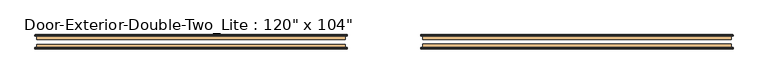
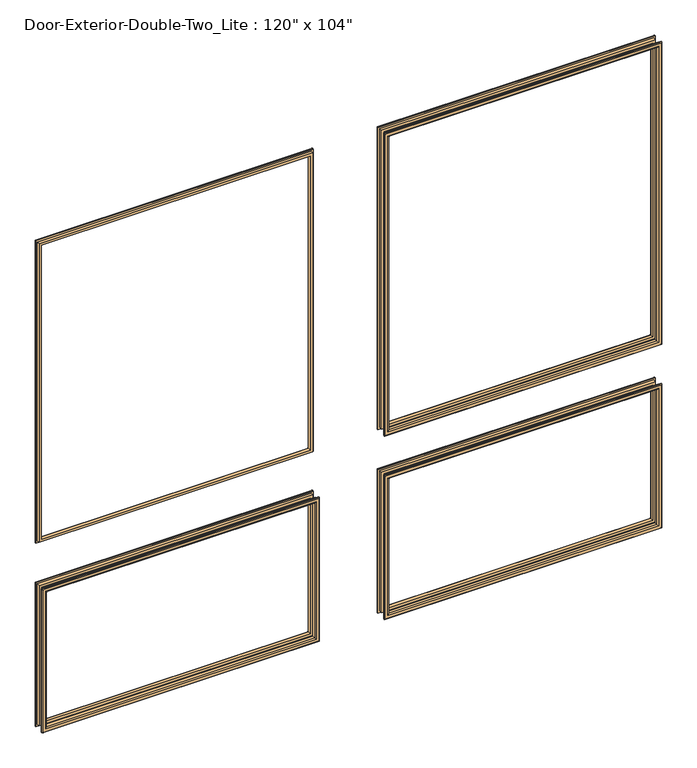
"""IFC4 building model written with IfcOpenShell, lengths in millimetres: door geometry."""

from ifc_helpers import new_model, si_unit, frame, origin, place, context, project, spatial, ellipse_curve, source, transform, mapped, element, save
from ifc_brep_helpers import plane_surface, cylinder_surface, advanced_brep


def door_e43601eb(model_context):
    return source(origin(), model_context, "Body", "AdvancedBrep", [
        advanced_brep(
        [(-1371.6, 69.85, 914.4), (-1371.6, 82.55, 914.4), (-1371.6, 82.55, 254.0), (-1371.6, 69.85, 254.0), (-1359.6, 83.55, 902.4), (-1359.6, 69.85, 902.4), (-1359.6, 69.85, 266.0), (-1359.6, 83.55, 266.0), (-1364.6, 88.55, 907.4), (-1364.6, 88.55, 261.0), (-1379.6, 86.55, 922.4), (-1377.6, 88.55, 920.4), (-1377.6, 88.55, 248.0), (-1379.6, 86.55, 246.0), (-1379.6, 82.55, 922.4), (-1379.6, 82.55, 246.0), (-152.4, 82.55, 254.0), (-152.4, 69.85, 254.0), (-164.4, 69.85, 266.0), (-164.4, 83.55, 266.0), (-159.4, 88.55, 261.0), (-146.4, 88.55, 248.0), (-144.4, 86.55, 246.0), (-144.4, 82.55, 246.0), (-152.4, 82.55, 914.4), (-152.4, 69.85, 914.4), (-164.4, 69.85, 902.4), (-164.4, 83.55, 902.4), (-159.4, 88.55, 907.4), (-146.4, 88.55, 920.4), (-144.4, 86.55, 922.4), (-144.4, 82.55, 922.4)],
        [
            (0, 1),
            (1, 2),
            (2, 3),
            (3, 0),
            (4, 5),
            (5, 6),
            (6, 7),
            (7, 4),
            (8, 4, ellipse_curve(frame((-1364.6, 83.55, 907.4), z_axis=(-0.7071067811865475, 0.0, -0.7071067811865475), x_axis=(-0.7071067811865474, 0.0, 0.7071067811865476)), 7.0710678, 5.0)),
            (7, 9, ellipse_curve(frame((-1364.6, 83.55, 261.0), z_axis=(-0.7071067811865475, 0.0, 0.7071067811865475), x_axis=(0.7071067811865474, 0.0, 0.7071067811865476)), 7.0710678, 5.0)),
            (9, 8),
            (10, 11, ellipse_curve(frame((-1377.6, 86.55, 920.4), z_axis=(-0.7071067811865475, 0.0, -0.7071067811865475), x_axis=(-0.7071067811865474, 0.0, 0.7071067811865476)), 2.8284271, 2.0)),
            (11, 12),
            (12, 13, ellipse_curve(frame((-1377.6, 86.55, 248.0), z_axis=(-0.7071067811865475, 0.0, 0.7071067811865475), x_axis=(0.7071067811865474, 0.0, 0.7071067811865476)), 2.8284271, 2.0)),
            (13, 10),
            (14, 10),
            (13, 15),
            (15, 14),
            (2, 16),
            (16, 17),
            (17, 3),
            (6, 18),
            (18, 19),
            (19, 7),
            (19, 20, ellipse_curve(frame((-159.4, 83.55, 261.0), z_axis=(-0.7071067811865475, 0.0, -0.7071067811865475), x_axis=(-0.7071067811865476, 0.0, 0.7071067811865474)), 7.0710678, 5.0)),
            (20, 9),
            (12, 21),
            (21, 22, ellipse_curve(frame((-146.4, 86.55, 248.0), z_axis=(-0.7071067811865475, 0.0, -0.7071067811865475), x_axis=(-0.7071067811865476, 0.0, 0.7071067811865474)), 2.8284271, 2.0)),
            (22, 13),
            (22, 23),
            (23, 15),
            (16, 24),
            (24, 25),
            (25, 17),
            (18, 26),
            (26, 27),
            (27, 19),
            (27, 28, ellipse_curve(frame((-159.4, 83.55, 907.4), z_axis=(0.7071067811865475, 0.0, -0.7071067811865475), x_axis=(-0.7071067811865474, 0.0, -0.7071067811865476)), 7.0710678, 5.0)),
            (28, 20),
            (21, 29),
            (29, 30, ellipse_curve(frame((-146.4, 86.55, 920.4), z_axis=(0.7071067811865475, 0.0, -0.7071067811865475), x_axis=(-0.7071067811865474, 0.0, -0.7071067811865476)), 2.8284271, 2.0)),
            (30, 22),
            (30, 31),
            (31, 23),
            (31, 14),
            (1, 24),
            (0, 25),
            (5, 26),
            (4, 27),
            (8, 28),
            (11, 29),
            (10, 30),
        ],
        [
            plane_surface(frame((-1371.6, 82.55, 914.4), z_axis=(-1.0, 0.0, 0.0), x_axis=(0.0, 0.0, -1.0))),
            plane_surface(frame((-1359.6, 69.85, 902.4), z_axis=(1.0, 0.0, 0.0), x_axis=(0.0, 0.0, -1.0))),
            cylinder_surface(frame((-1364.6, 83.55, 914.4), z_axis=(0.0, 0.0, 1.0), x_axis=(-1.0, 0.0, 0.0)), 5.0),
            cylinder_surface(frame((-1377.6, 86.55, 914.4), z_axis=(0.0, 0.0, 1.0), x_axis=(-1.0, 0.0, 0.0)), 2.0),
            plane_surface(frame((-1379.6, 86.55, 922.4), z_axis=(-1.0, 0.0, 0.0), x_axis=(0.0, 0.0, -1.0))),
            plane_surface(frame((-1371.6, 82.55, 254.0), z_axis=(0.0, 0.0, -1.0), x_axis=(1.0, 0.0, 0.0))),
            plane_surface(frame((-1359.6, 69.85, 266.0), z_axis=(0.0, 0.0, 1.0), x_axis=(1.0, 0.0, 0.0))),
            cylinder_surface(frame((-1371.6, 83.55, 261.0), z_axis=(-1.0, 0.0, 0.0), x_axis=(0.0, 0.0, -1.0)), 5.0),
            cylinder_surface(frame((-1371.6, 86.55, 248.0), z_axis=(-1.0, 0.0, 0.0), x_axis=(0.0, 0.0, -1.0)), 2.0),
            plane_surface(frame((-1379.6, 86.55, 246.0), z_axis=(0.0, 0.0, -1.0), x_axis=(1.0, 0.0, 0.0))),
            plane_surface(frame((-152.4, 82.55, 254.0), z_axis=(1.0, 0.0, 0.0), x_axis=(0.0, 0.0, 1.0))),
            plane_surface(frame((-164.4, 69.85, 266.0), z_axis=(-1.0, 0.0, 0.0), x_axis=(0.0, 0.0, 1.0))),
            cylinder_surface(frame((-159.4, 83.55, 254.0), z_axis=(0.0, 0.0, -1.0), x_axis=(1.0, 0.0, 0.0)), 5.0),
            cylinder_surface(frame((-146.4, 86.55, 254.0), z_axis=(0.0, 0.0, -1.0), x_axis=(1.0, 0.0, 0.0)), 2.0),
            plane_surface(frame((-144.4, 86.55, 246.0), z_axis=(1.0, 0.0, 0.0), x_axis=(0.0, 0.0, 1.0))),
            plane_surface(frame((-144.4, 82.55, 922.4), z_axis=(0.0, -1.0, 0.0), x_axis=(-1.0, 0.0, 0.0))),
            plane_surface(frame((-152.4, 82.55, 914.4), z_axis=(0.0, 0.0, 1.0), x_axis=(-1.0, 0.0, 0.0))),
            plane_surface(frame((-152.4, 69.85, 914.4), z_axis=(0.0, -1.0, 0.0), x_axis=(-1.0, 0.0, 0.0))),
            plane_surface(frame((-164.4, 69.85, 902.4), z_axis=(0.0, 0.0, -1.0), x_axis=(-1.0, 0.0, 0.0))),
            cylinder_surface(frame((-152.4, 83.55, 907.4), z_axis=(1.0, 0.0, 0.0), x_axis=(0.0, 0.0, 1.0)), 5.0),
            plane_surface(frame((-159.4, 88.55, 907.4), z_axis=(0.0, 1.0, 0.0), x_axis=(-1.0, 0.0, 0.0))),
            cylinder_surface(frame((-152.4, 86.55, 920.4), z_axis=(1.0, 0.0, 0.0), x_axis=(0.0, 0.0, 1.0)), 2.0),
            plane_surface(frame((-144.4, 86.55, 922.4), z_axis=(0.0, 0.0, 1.0), x_axis=(-1.0, 0.0, 0.0))),
        ],
        [
            (0, [[1, 2, 3, 4]]),
            (1, [[5, 6, 7, 8]]),
            (2, [[9, -8, 10, 11]]),
            (3, [[12, 13, 14, 15]]),
            (4, [[16, -15, 17, 18]]),
            (5, [[-3, 19, 20, 21]]),
            (6, [[-7, 22, 23, 24]]),
            (7, [[-10, -24, 25, 26]]),
            (8, [[-14, 27, 28, 29]]),
            (9, [[-17, -29, 30, 31]]),
            (10, [[-20, 32, 33, 34]]),
            (11, [[-23, 35, 36, 37]]),
            (12, [[-25, -37, 38, 39]]),
            (13, [[-28, 40, 41, 42]]),
            (14, [[-30, -42, 43, 44]]),
            (15, [[-31, -44, 45, -18], [46, -32, -19, -2]]),
            (16, [[-33, -46, -1, 47]]),
            (17, [[-21, -34, -47, -4], [48, -35, -22, -6]]),
            (18, [[-36, -48, -5, 49]]),
            (19, [[-38, -49, -9, 50]]),
            (20, [[51, -40, -27, -13], [-26, -39, -50, -11]]),
            (21, [[-41, -51, -12, 52]]),
            (22, [[-43, -52, -16, -45]]),
        ],
    ),
        advanced_brep(
        [(152.4, 69.85, 914.4), (152.4, 82.55, 914.4), (152.4, 82.55, 254.0), (152.4, 69.85, 254.0), (164.4, 83.55, 902.4), (164.4, 69.85, 902.4), (164.4, 69.85, 266.0), (164.4, 83.55, 266.0), (159.4, 88.55, 907.4), (159.4, 88.55, 261.0), (144.4, 86.55, 922.4), (146.4, 88.55, 920.4), (146.4, 88.55, 248.0), (144.4, 86.55, 246.0), (144.4, 82.55, 922.4), (144.4, 82.55, 246.0), (1371.6, 82.55, 254.0), (1371.6, 69.85, 254.0), (1359.6, 69.85, 266.0), (1359.6, 83.55, 266.0), (1364.6, 88.55, 261.0), (1377.6, 88.55, 248.0), (1379.6, 86.55, 246.0), (1379.6, 82.55, 246.0), (1371.6, 82.55, 914.4), (1371.6, 69.85, 914.4), (1359.6, 69.85, 902.4), (1359.6, 83.55, 902.4), (1364.6, 88.55, 907.4), (1377.6, 88.55, 920.4), (1379.6, 86.55, 922.4), (1379.6, 82.55, 922.4)],
        [
            (0, 1),
            (1, 2),
            (2, 3),
            (3, 0),
            (4, 5),
            (5, 6),
            (6, 7),
            (7, 4),
            (8, 4, ellipse_curve(frame((159.4, 83.55, 907.4), z_axis=(-0.7071067811865475, 0.0, -0.7071067811865475), x_axis=(-0.7071067811865474, 0.0, 0.7071067811865476)), 7.0710678, 5.0)),
            (7, 9, ellipse_curve(frame((159.4, 83.55, 261.0), z_axis=(-0.7071067811865475, 0.0, 0.7071067811865475), x_axis=(0.7071067811865474, 0.0, 0.7071067811865476)), 7.0710678, 5.0)),
            (9, 8),
            (10, 11, ellipse_curve(frame((146.4, 86.55, 920.4), z_axis=(-0.7071067811865475, 0.0, -0.7071067811865475), x_axis=(-0.7071067811865474, 0.0, 0.7071067811865476)), 2.8284271, 2.0)),
            (11, 12),
            (12, 13, ellipse_curve(frame((146.4, 86.55, 248.0), z_axis=(-0.7071067811865475, 0.0, 0.7071067811865475), x_axis=(0.7071067811865474, 0.0, 0.7071067811865476)), 2.8284271, 2.0)),
            (13, 10),
            (14, 10),
            (13, 15),
            (15, 14),
            (2, 16),
            (16, 17),
            (17, 3),
            (6, 18),
            (18, 19),
            (19, 7),
            (19, 20, ellipse_curve(frame((1364.6, 83.55, 261.0), z_axis=(-0.7071067811865475, 0.0, -0.7071067811865475), x_axis=(-0.7071067811865476, 0.0, 0.7071067811865474)), 7.0710678, 5.0)),
            (20, 9),
            (12, 21),
            (21, 22, ellipse_curve(frame((1377.6, 86.55, 248.0), z_axis=(-0.7071067811865475, 0.0, -0.7071067811865475), x_axis=(-0.7071067811865476, 0.0, 0.7071067811865474)), 2.8284271, 2.0)),
            (22, 13),
            (22, 23),
            (23, 15),
            (16, 24),
            (24, 25),
            (25, 17),
            (18, 26),
            (26, 27),
            (27, 19),
            (27, 28, ellipse_curve(frame((1364.6, 83.55, 907.4), z_axis=(0.7071067811865475, 0.0, -0.7071067811865475), x_axis=(-0.7071067811865474, 0.0, -0.7071067811865476)), 7.0710678, 5.0)),
            (28, 20),
            (21, 29),
            (29, 30, ellipse_curve(frame((1377.6, 86.55, 920.4), z_axis=(0.7071067811865475, 0.0, -0.7071067811865475), x_axis=(-0.7071067811865474, 0.0, -0.7071067811865476)), 2.8284271, 2.0)),
            (30, 22),
            (30, 31),
            (31, 23),
            (31, 14),
            (1, 24),
            (0, 25),
            (5, 26),
            (4, 27),
            (8, 28),
            (11, 29),
            (10, 30),
        ],
        [
            plane_surface(frame((152.4, 82.55, 914.4), z_axis=(-1.0, 0.0, 0.0), x_axis=(0.0, 0.0, -1.0))),
            plane_surface(frame((164.4, 69.85, 902.4), z_axis=(1.0, 0.0, 0.0), x_axis=(0.0, 0.0, -1.0))),
            cylinder_surface(frame((159.4, 83.55, 914.4), z_axis=(0.0, 0.0, 1.0), x_axis=(-1.0, 0.0, 0.0)), 5.0),
            cylinder_surface(frame((146.4, 86.55, 914.4), z_axis=(0.0, 0.0, 1.0), x_axis=(-1.0, 0.0, 0.0)), 2.0),
            plane_surface(frame((144.4, 86.55, 922.4), z_axis=(-1.0, 0.0, 0.0), x_axis=(0.0, 0.0, -1.0))),
            plane_surface(frame((152.4, 82.55, 254.0), z_axis=(0.0, 0.0, -1.0), x_axis=(1.0, 0.0, 0.0))),
            plane_surface(frame((164.4, 69.85, 266.0), z_axis=(0.0, 0.0, 1.0), x_axis=(1.0, 0.0, 0.0))),
            cylinder_surface(frame((152.4, 83.55, 261.0), z_axis=(-1.0, 0.0, 0.0), x_axis=(0.0, 0.0, -1.0)), 5.0),
            cylinder_surface(frame((152.4, 86.55, 248.0), z_axis=(-1.0, 0.0, 0.0), x_axis=(0.0, 0.0, -1.0)), 2.0),
            plane_surface(frame((144.4, 86.55, 246.0), z_axis=(0.0, 0.0, -1.0), x_axis=(1.0, 0.0, 0.0))),
            plane_surface(frame((1371.6, 82.55, 254.0), z_axis=(1.0, 0.0, 0.0), x_axis=(0.0, 0.0, 1.0))),
            plane_surface(frame((1359.6, 69.85, 266.0), z_axis=(-1.0, 0.0, 0.0), x_axis=(0.0, 0.0, 1.0))),
            cylinder_surface(frame((1364.6, 83.55, 254.0), z_axis=(0.0, 0.0, -1.0), x_axis=(1.0, 0.0, 0.0)), 5.0),
            cylinder_surface(frame((1377.6, 86.55, 254.0), z_axis=(0.0, 0.0, -1.0), x_axis=(1.0, 0.0, 0.0)), 2.0),
            plane_surface(frame((1379.6, 86.55, 246.0), z_axis=(1.0, 0.0, 0.0), x_axis=(0.0, 0.0, 1.0))),
            plane_surface(frame((1379.6, 82.55, 922.4), z_axis=(0.0, -1.0, 0.0), x_axis=(-1.0, 0.0, 0.0))),
            plane_surface(frame((1371.6, 82.55, 914.4), z_axis=(0.0, 0.0, 1.0), x_axis=(-1.0, 0.0, 0.0))),
            plane_surface(frame((1371.6, 69.85, 914.4), z_axis=(0.0, -1.0, 0.0), x_axis=(-1.0, 0.0, 0.0))),
            plane_surface(frame((1359.6, 69.85, 902.4), z_axis=(0.0, 0.0, -1.0), x_axis=(-1.0, 0.0, 0.0))),
            cylinder_surface(frame((1371.6, 83.55, 907.4), z_axis=(1.0, 0.0, 0.0), x_axis=(0.0, 0.0, 1.0)), 5.0),
            plane_surface(frame((1364.6, 88.55, 907.4), z_axis=(0.0, 1.0, 0.0), x_axis=(-1.0, 0.0, 0.0))),
            cylinder_surface(frame((1371.6, 86.55, 920.4), z_axis=(1.0, 0.0, 0.0), x_axis=(0.0, 0.0, 1.0)), 2.0),
            plane_surface(frame((1379.6, 86.55, 922.4), z_axis=(0.0, 0.0, 1.0), x_axis=(-1.0, 0.0, 0.0))),
        ],
        [
            (0, [[1, 2, 3, 4]]),
            (1, [[5, 6, 7, 8]]),
            (2, [[9, -8, 10, 11]]),
            (3, [[12, 13, 14, 15]]),
            (4, [[16, -15, 17, 18]]),
            (5, [[-3, 19, 20, 21]]),
            (6, [[-7, 22, 23, 24]]),
            (7, [[-10, -24, 25, 26]]),
            (8, [[-14, 27, 28, 29]]),
            (9, [[-17, -29, 30, 31]]),
            (10, [[-20, 32, 33, 34]]),
            (11, [[-23, 35, 36, 37]]),
            (12, [[-25, -37, 38, 39]]),
            (13, [[-28, 40, 41, 42]]),
            (14, [[-30, -42, 43, 44]]),
            (15, [[-31, -44, 45, -18], [46, -32, -19, -2]]),
            (16, [[-33, -46, -1, 47]]),
            (17, [[-21, -34, -47, -4], [48, -35, -22, -6]]),
            (18, [[-36, -48, -5, 49]]),
            (19, [[-38, -49, -9, 50]]),
            (20, [[51, -40, -27, -13], [-26, -39, -50, -11]]),
            (21, [[-41, -51, -12, 52]]),
            (22, [[-43, -52, -16, -45]]),
        ],
    ),
        advanced_brep(
        [(152.4, 69.85, 2524.125), (152.4, 82.55, 2524.125), (152.4, 82.55, 1117.6), (152.4, 69.85, 1117.6), (164.4, 83.55, 2512.125), (164.4, 69.85, 2512.125), (164.4, 69.85, 1129.6), (164.4, 83.55, 1129.6), (159.4, 88.55, 2517.125), (159.4, 88.55, 1124.6), (144.4, 86.55, 2532.125), (146.4, 88.55, 2530.125), (146.4, 88.55, 1111.6), (144.4, 86.55, 1109.6), (144.4, 82.55, 2532.125), (144.4, 82.55, 1109.6), (1371.6, 82.55, 1117.6), (1371.6, 69.85, 1117.6), (1359.6, 69.85, 1129.6), (1359.6, 83.55, 1129.6), (1364.6, 88.55, 1124.6), (1377.6, 88.55, 1111.6), (1379.6, 86.55, 1109.6), (1379.6, 82.55, 1109.6), (1371.6, 82.55, 2524.125), (1371.6, 69.85, 2524.125), (1359.6, 69.85, 2512.125), (1359.6, 83.55, 2512.125), (1364.6, 88.55, 2517.125), (1377.6, 88.55, 2530.125), (1379.6, 86.55, 2532.125), (1379.6, 82.55, 2532.125)],
        [
            (0, 1),
            (1, 2),
            (2, 3),
            (3, 0),
            (4, 5),
            (5, 6),
            (6, 7),
            (7, 4),
            (8, 4, ellipse_curve(frame((159.4, 83.55, 2517.125), z_axis=(-0.7071067811865475, 0.0, -0.7071067811865475), x_axis=(-0.7071067811865474, 0.0, 0.7071067811865476)), 7.0710678, 5.0)),
            (7, 9, ellipse_curve(frame((159.4, 83.55, 1124.6), z_axis=(-0.7071067811865475, 0.0, 0.7071067811865475), x_axis=(0.7071067811865474, 0.0, 0.7071067811865476)), 7.0710678, 5.0)),
            (9, 8),
            (10, 11, ellipse_curve(frame((146.4, 86.55, 2530.125), z_axis=(-0.7071067811865475, 0.0, -0.7071067811865475), x_axis=(-0.7071067811865474, 0.0, 0.7071067811865476)), 2.8284271, 2.0)),
            (11, 12),
            (12, 13, ellipse_curve(frame((146.4, 86.55, 1111.6), z_axis=(-0.7071067811865475, 0.0, 0.7071067811865475), x_axis=(0.7071067811865474, 0.0, 0.7071067811865476)), 2.8284271, 2.0)),
            (13, 10),
            (14, 10),
            (13, 15),
            (15, 14),
            (2, 16),
            (16, 17),
            (17, 3),
            (6, 18),
            (18, 19),
            (19, 7),
            (19, 20, ellipse_curve(frame((1364.6, 83.55, 1124.6), z_axis=(-0.7071067811865475, 0.0, -0.7071067811865475), x_axis=(-0.7071067811865476, 0.0, 0.7071067811865474)), 7.0710678, 5.0)),
            (20, 9),
            (12, 21),
            (21, 22, ellipse_curve(frame((1377.6, 86.55, 1111.6), z_axis=(-0.7071067811865475, 0.0, -0.7071067811865475), x_axis=(-0.7071067811865476, 0.0, 0.7071067811865474)), 2.8284271, 2.0)),
            (22, 13),
            (22, 23),
            (23, 15),
            (16, 24),
            (24, 25),
            (25, 17),
            (18, 26),
            (26, 27),
            (27, 19),
            (27, 28, ellipse_curve(frame((1364.6, 83.55, 2517.125), z_axis=(0.7071067811865475, 0.0, -0.7071067811865475), x_axis=(-0.7071067811865474, 0.0, -0.7071067811865476)), 7.0710678, 5.0)),
            (28, 20),
            (21, 29),
            (29, 30, ellipse_curve(frame((1377.6, 86.55, 2530.125), z_axis=(0.7071067811865475, 0.0, -0.7071067811865475), x_axis=(-0.7071067811865474, 0.0, -0.7071067811865476)), 2.8284271, 2.0)),
            (30, 22),
            (30, 31),
            (31, 23),
            (31, 14),
            (1, 24),
            (0, 25),
            (5, 26),
            (4, 27),
            (8, 28),
            (11, 29),
            (10, 30),
        ],
        [
            plane_surface(frame((152.4, 82.55, 2524.125), z_axis=(-1.0, 0.0, 0.0), x_axis=(0.0, 0.0, -1.0))),
            plane_surface(frame((164.4, 69.85, 2512.125), z_axis=(1.0, 0.0, 0.0), x_axis=(0.0, 0.0, -1.0))),
            cylinder_surface(frame((159.4, 83.55, 2524.125), z_axis=(0.0, 0.0, 1.0), x_axis=(-1.0, 0.0, 0.0)), 5.0),
            cylinder_surface(frame((146.4, 86.55, 2524.125), z_axis=(0.0, 0.0, 1.0), x_axis=(-1.0, 0.0, 0.0)), 2.0),
            plane_surface(frame((144.4, 86.55, 2532.125), z_axis=(-1.0, 0.0, 0.0), x_axis=(0.0, 0.0, -1.0))),
            plane_surface(frame((152.4, 82.55, 1117.6), z_axis=(0.0, 0.0, -1.0), x_axis=(1.0, 0.0, 0.0))),
            plane_surface(frame((164.4, 69.85, 1129.6), z_axis=(0.0, 0.0, 1.0), x_axis=(1.0, 0.0, 0.0))),
            cylinder_surface(frame((152.4, 83.55, 1124.6), z_axis=(-1.0, 0.0, 0.0), x_axis=(0.0, 0.0, -1.0)), 5.0),
            cylinder_surface(frame((152.4, 86.55, 1111.6), z_axis=(-1.0, 0.0, 0.0), x_axis=(0.0, 0.0, -1.0)), 2.0),
            plane_surface(frame((144.4, 86.55, 1109.6), z_axis=(0.0, 0.0, -1.0), x_axis=(1.0, 0.0, 0.0))),
            plane_surface(frame((1371.6, 82.55, 1117.6), z_axis=(1.0, 0.0, 0.0), x_axis=(0.0, 0.0, 1.0))),
            plane_surface(frame((1359.6, 69.85, 1129.6), z_axis=(-1.0, 0.0, 0.0), x_axis=(0.0, 0.0, 1.0))),
            cylinder_surface(frame((1364.6, 83.55, 1117.6), z_axis=(0.0, 0.0, -1.0), x_axis=(1.0, 0.0, 0.0)), 5.0),
            cylinder_surface(frame((1377.6, 86.55, 1117.6), z_axis=(0.0, 0.0, -1.0), x_axis=(1.0, 0.0, 0.0)), 2.0),
            plane_surface(frame((1379.6, 86.55, 1109.6), z_axis=(1.0, 0.0, 0.0), x_axis=(0.0, 0.0, 1.0))),
            plane_surface(frame((1379.6, 82.55, 2532.125), z_axis=(0.0, -1.0, 0.0), x_axis=(-1.0, 0.0, 0.0))),
            plane_surface(frame((1371.6, 82.55, 2524.125), z_axis=(0.0, 0.0, 1.0), x_axis=(-1.0, 0.0, 0.0))),
            plane_surface(frame((1371.6, 69.85, 2524.125), z_axis=(0.0, -1.0, 0.0), x_axis=(-1.0, 0.0, 0.0))),
            plane_surface(frame((1359.6, 69.85, 2512.125), z_axis=(0.0, 0.0, -1.0), x_axis=(-1.0, 0.0, 0.0))),
            cylinder_surface(frame((1371.6, 83.55, 2517.125), z_axis=(1.0, 0.0, 0.0), x_axis=(0.0, 0.0, 1.0)), 5.0),
            plane_surface(frame((1364.6, 88.55, 2517.125), z_axis=(0.0, 1.0, 0.0), x_axis=(-1.0, 0.0, 0.0))),
            cylinder_surface(frame((1371.6, 86.55, 2530.125), z_axis=(1.0, 0.0, 0.0), x_axis=(0.0, 0.0, 1.0)), 2.0),
            plane_surface(frame((1379.6, 86.55, 2532.125), z_axis=(0.0, 0.0, 1.0), x_axis=(-1.0, 0.0, 0.0))),
        ],
        [
            (0, [[1, 2, 3, 4]]),
            (1, [[5, 6, 7, 8]]),
            (2, [[9, -8, 10, 11]]),
            (3, [[12, 13, 14, 15]]),
            (4, [[16, -15, 17, 18]]),
            (5, [[-3, 19, 20, 21]]),
            (6, [[-7, 22, 23, 24]]),
            (7, [[-10, -24, 25, 26]]),
            (8, [[-14, 27, 28, 29]]),
            (9, [[-17, -29, 30, 31]]),
            (10, [[-20, 32, 33, 34]]),
            (11, [[-23, 35, 36, 37]]),
            (12, [[-25, -37, 38, 39]]),
            (13, [[-28, 40, 41, 42]]),
            (14, [[-30, -42, 43, 44]]),
            (15, [[-31, -44, 45, -18], [46, -32, -19, -2]]),
            (16, [[-33, -46, -1, 47]]),
            (17, [[-21, -34, -47, -4], [48, -35, -22, -6]]),
            (18, [[-36, -48, -5, 49]]),
            (19, [[-38, -49, -9, 50]]),
            (20, [[51, -40, -27, -13], [-26, -39, -50, -11]]),
            (21, [[-41, -51, -12, 52]]),
            (22, [[-43, -52, -16, -45]]),
        ],
    ),
        advanced_brep(
        [(-1371.6, 69.85, 2524.125), (-1371.6, 82.55, 2524.125), (-1371.6, 82.55, 1117.6), (-1371.6, 69.85, 1117.6), (-1359.6, 83.55, 2512.125), (-1359.6, 69.85, 2512.125), (-1359.6, 69.85, 1129.6), (-1359.6, 83.55, 1129.6), (-1364.6, 88.55, 2517.125), (-1364.6, 88.55, 1124.6), (-1379.6, 86.55, 2532.125), (-1377.6, 88.55, 2530.125), (-1377.6, 88.55, 1111.6), (-1379.6, 86.55, 1109.6), (-1379.6, 82.55, 2532.125), (-1379.6, 82.55, 1109.6), (-152.4, 82.55, 1117.6), (-152.4, 69.85, 1117.6), (-164.4, 69.85, 1129.6), (-164.4, 83.55, 1129.6), (-159.4, 88.55, 1124.6), (-146.4, 88.55, 1111.6), (-144.4, 86.55, 1109.6), (-144.4, 82.55, 1109.6), (-152.4, 82.55, 2524.125), (-152.4, 69.85, 2524.125), (-164.4, 69.85, 2512.125), (-164.4, 83.55, 2512.125), (-159.4, 88.55, 2517.125), (-146.4, 88.55, 2530.125), (-144.4, 86.55, 2532.125), (-144.4, 82.55, 2532.125)],
        [
            (0, 1),
            (1, 2),
            (2, 3),
            (3, 0),
            (4, 5),
            (5, 6),
            (6, 7),
            (7, 4),
            (8, 4, ellipse_curve(frame((-1364.6, 83.55, 2517.125), z_axis=(-0.7071067811865475, 0.0, -0.7071067811865475), x_axis=(-0.7071067811865474, 0.0, 0.7071067811865476)), 7.0710678, 5.0)),
            (7, 9, ellipse_curve(frame((-1364.6, 83.55, 1124.6), z_axis=(-0.7071067811865475, 0.0, 0.7071067811865475), x_axis=(0.7071067811865474, 0.0, 0.7071067811865476)), 7.0710678, 5.0)),
            (9, 8),
            (10, 11, ellipse_curve(frame((-1377.6, 86.55, 2530.125), z_axis=(-0.7071067811865475, 0.0, -0.7071067811865475), x_axis=(-0.7071067811865474, 0.0, 0.7071067811865476)), 2.8284271, 2.0)),
            (11, 12),
            (12, 13, ellipse_curve(frame((-1377.6, 86.55, 1111.6), z_axis=(-0.7071067811865475, 0.0, 0.7071067811865475), x_axis=(0.7071067811865474, 0.0, 0.7071067811865476)), 2.8284271, 2.0)),
            (13, 10),
            (14, 10),
            (13, 15),
            (15, 14),
            (2, 16),
            (16, 17),
            (17, 3),
            (6, 18),
            (18, 19),
            (19, 7),
            (19, 20, ellipse_curve(frame((-159.4, 83.55, 1124.6), z_axis=(-0.7071067811865475, 0.0, -0.7071067811865475), x_axis=(-0.7071067811865476, 0.0, 0.7071067811865474)), 7.0710678, 5.0)),
            (20, 9),
            (12, 21),
            (21, 22, ellipse_curve(frame((-146.4, 86.55, 1111.6), z_axis=(-0.7071067811865475, 0.0, -0.7071067811865475), x_axis=(-0.7071067811865476, 0.0, 0.7071067811865474)), 2.8284271, 2.0)),
            (22, 13),
            (22, 23),
            (23, 15),
            (16, 24),
            (24, 25),
            (25, 17),
            (18, 26),
            (26, 27),
            (27, 19),
            (27, 28, ellipse_curve(frame((-159.4, 83.55, 2517.125), z_axis=(0.7071067811865475, 0.0, -0.7071067811865475), x_axis=(-0.7071067811865474, 0.0, -0.7071067811865476)), 7.0710678, 5.0)),
            (28, 20),
            (21, 29),
            (29, 30, ellipse_curve(frame((-146.4, 86.55, 2530.125), z_axis=(0.7071067811865475, 0.0, -0.7071067811865475), x_axis=(-0.7071067811865474, 0.0, -0.7071067811865476)), 2.8284271, 2.0)),
            (30, 22),
            (30, 31),
            (31, 23),
            (31, 14),
            (1, 24),
            (0, 25),
            (5, 26),
            (4, 27),
            (8, 28),
            (11, 29),
            (10, 30),
        ],
        [
            plane_surface(frame((-1371.6, 82.55, 2524.125), z_axis=(-1.0, 0.0, 0.0), x_axis=(0.0, 0.0, -1.0))),
            plane_surface(frame((-1359.6, 69.85, 2512.125), z_axis=(1.0, 0.0, 0.0), x_axis=(0.0, 0.0, -1.0))),
            cylinder_surface(frame((-1364.6, 83.55, 2524.125), z_axis=(0.0, 0.0, 1.0), x_axis=(-1.0, 0.0, 0.0)), 5.0),
            cylinder_surface(frame((-1377.6, 86.55, 2524.125), z_axis=(0.0, 0.0, 1.0), x_axis=(-1.0, 0.0, 0.0)), 2.0),
            plane_surface(frame((-1379.6, 86.55, 2532.125), z_axis=(-1.0, 0.0, 0.0), x_axis=(0.0, 0.0, -1.0))),
            plane_surface(frame((-1371.6, 82.55, 1117.6), z_axis=(0.0, 0.0, -1.0), x_axis=(1.0, 0.0, 0.0))),
            plane_surface(frame((-1359.6, 69.85, 1129.6), z_axis=(0.0, 0.0, 1.0), x_axis=(1.0, 0.0, 0.0))),
            cylinder_surface(frame((-1371.6, 83.55, 1124.6), z_axis=(-1.0, 0.0, 0.0), x_axis=(0.0, 0.0, -1.0)), 5.0),
            cylinder_surface(frame((-1371.6, 86.55, 1111.6), z_axis=(-1.0, 0.0, 0.0), x_axis=(0.0, 0.0, -1.0)), 2.0),
            plane_surface(frame((-1379.6, 86.55, 1109.6), z_axis=(0.0, 0.0, -1.0), x_axis=(1.0, 0.0, 0.0))),
            plane_surface(frame((-152.4, 82.55, 1117.6), z_axis=(1.0, 0.0, 0.0), x_axis=(0.0, 0.0, 1.0))),
            plane_surface(frame((-164.4, 69.85, 1129.6), z_axis=(-1.0, 0.0, 0.0), x_axis=(0.0, 0.0, 1.0))),
            cylinder_surface(frame((-159.4, 83.55, 1117.6), z_axis=(0.0, 0.0, -1.0), x_axis=(1.0, 0.0, 0.0)), 5.0),
            cylinder_surface(frame((-146.4, 86.55, 1117.6), z_axis=(0.0, 0.0, -1.0), x_axis=(1.0, 0.0, 0.0)), 2.0),
            plane_surface(frame((-144.4, 86.55, 1109.6), z_axis=(1.0, 0.0, 0.0), x_axis=(0.0, 0.0, 1.0))),
            plane_surface(frame((-144.4, 82.55, 2532.125), z_axis=(0.0, -1.0, 0.0), x_axis=(-1.0, 0.0, 0.0))),
            plane_surface(frame((-152.4, 82.55, 2524.125), z_axis=(0.0, 0.0, 1.0), x_axis=(-1.0, 0.0, 0.0))),
            plane_surface(frame((-152.4, 69.85, 2524.125), z_axis=(0.0, -1.0, 0.0), x_axis=(-1.0, 0.0, 0.0))),
            plane_surface(frame((-164.4, 69.85, 2512.125), z_axis=(0.0, 0.0, -1.0), x_axis=(-1.0, 0.0, 0.0))),
            cylinder_surface(frame((-152.4, 83.55, 2517.125), z_axis=(1.0, 0.0, 0.0), x_axis=(0.0, 0.0, 1.0)), 5.0),
            plane_surface(frame((-159.4, 88.55, 2517.125), z_axis=(0.0, 1.0, 0.0), x_axis=(-1.0, 0.0, 0.0))),
            cylinder_surface(frame((-152.4, 86.55, 2530.125), z_axis=(1.0, 0.0, 0.0), x_axis=(0.0, 0.0, 1.0)), 2.0),
            plane_surface(frame((-144.4, 86.55, 2532.125), z_axis=(0.0, 0.0, 1.0), x_axis=(-1.0, 0.0, 0.0))),
        ],
        [
            (0, [[1, 2, 3, 4]]),
            (1, [[5, 6, 7, 8]]),
            (2, [[9, -8, 10, 11]]),
            (3, [[12, 13, 14, 15]]),
            (4, [[16, -15, 17, 18]]),
            (5, [[-3, 19, 20, 21]]),
            (6, [[-7, 22, 23, 24]]),
            (7, [[-10, -24, 25, 26]]),
            (8, [[-14, 27, 28, 29]]),
            (9, [[-17, -29, 30, 31]]),
            (10, [[-20, 32, 33, 34]]),
            (11, [[-23, 35, 36, 37]]),
            (12, [[-25, -37, 38, 39]]),
            (13, [[-28, 40, 41, 42]]),
            (14, [[-30, -42, 43, 44]]),
            (15, [[-31, -44, 45, -18], [46, -32, -19, -2]]),
            (16, [[-33, -46, -1, 47]]),
            (17, [[-21, -34, -47, -4], [48, -35, -22, -6]]),
            (18, [[-36, -48, -5, 49]]),
            (19, [[-38, -49, -9, 50]]),
            (20, [[51, -40, -27, -13], [-26, -39, -50, -11]]),
            (21, [[-41, -51, -12, 52]]),
            (22, [[-43, -52, -16, -45]]),
        ],
    ),
        advanced_brep(
        [(-1371.6, 50.8, 254.0), (-1371.6, 38.1, 254.0), (-1371.6, 38.1, 914.4), (-1371.6, 50.8, 914.4), (-1359.6, 37.1, 266.0), (-1359.6, 50.8, 266.0), (-1359.6, 50.8, 902.4), (-1359.6, 37.1, 902.4), (-1364.6, 32.1, 261.0), (-1364.6, 32.1, 907.4), (-1379.6, 34.1, 246.0), (-1377.6, 32.1, 248.0), (-1377.6, 32.1, 920.4), (-1379.6, 34.1, 922.4), (-1379.6, 38.1, 246.0), (-1379.6, 38.1, 922.4), (-152.4, 38.1, 914.4), (-152.4, 50.8, 914.4), (-164.4, 50.8, 902.4), (-164.4, 37.1, 902.4), (-159.4, 32.1, 907.4), (-146.4, 32.1, 920.4), (-144.4, 34.1, 922.4), (-144.4, 38.1, 922.4), (-152.4, 38.1, 254.0), (-152.4, 50.8, 254.0), (-164.4, 50.8, 266.0), (-164.4, 37.1, 266.0), (-159.4, 32.1, 261.0), (-146.4, 32.1, 248.0), (-144.4, 34.1, 246.0), (-144.4, 38.1, 246.0)],
        [
            (0, 1),
            (1, 2),
            (2, 3),
            (3, 0),
            (4, 5),
            (5, 6),
            (6, 7),
            (7, 4),
            (8, 4, ellipse_curve(frame((-1364.6, 37.1, 261.0), z_axis=(-0.7071067811865475, 0.0, 0.7071067811865475), x_axis=(-0.7071067811865474, 0.0, -0.7071067811865476)), 7.0710678, 5.0)),
            (7, 9, ellipse_curve(frame((-1364.6, 37.1, 907.4), z_axis=(-0.7071067811865475, 0.0, -0.7071067811865475), x_axis=(0.7071067811865474, 0.0, -0.7071067811865476)), 7.0710678, 5.0)),
            (9, 8),
            (10, 11, ellipse_curve(frame((-1377.6, 34.1, 248.0), z_axis=(-0.7071067811865475, 0.0, 0.7071067811865475), x_axis=(-0.7071067811865474, 0.0, -0.7071067811865476)), 2.8284271, 2.0)),
            (11, 12),
            (12, 13, ellipse_curve(frame((-1377.6, 34.1, 920.4), z_axis=(-0.7071067811865475, 0.0, -0.7071067811865475), x_axis=(0.7071067811865474, 0.0, -0.7071067811865476)), 2.8284271, 2.0)),
            (13, 10),
            (14, 10),
            (13, 15),
            (15, 14),
            (2, 16),
            (16, 17),
            (17, 3),
            (6, 18),
            (18, 19),
            (19, 7),
            (19, 20, ellipse_curve(frame((-159.4, 37.1, 907.4), z_axis=(-0.7071067811865475, 0.0, 0.7071067811865475), x_axis=(-0.7071067811865476, 0.0, -0.7071067811865474)), 7.0710678, 5.0)),
            (20, 9),
            (12, 21),
            (21, 22, ellipse_curve(frame((-146.4, 34.1, 920.4), z_axis=(-0.7071067811865475, 0.0, 0.7071067811865475), x_axis=(-0.7071067811865476, 0.0, -0.7071067811865474)), 2.8284271, 2.0)),
            (22, 13),
            (22, 23),
            (23, 15),
            (16, 24),
            (24, 25),
            (25, 17),
            (18, 26),
            (26, 27),
            (27, 19),
            (27, 28, ellipse_curve(frame((-159.4, 37.1, 261.0), z_axis=(0.7071067811865475, 0.0, 0.7071067811865475), x_axis=(-0.7071067811865474, 0.0, 0.7071067811865476)), 7.0710678, 5.0)),
            (28, 20),
            (21, 29),
            (29, 30, ellipse_curve(frame((-146.4, 34.1, 248.0), z_axis=(0.7071067811865475, 0.0, 0.7071067811865475), x_axis=(-0.7071067811865474, 0.0, 0.7071067811865476)), 2.8284271, 2.0)),
            (30, 22),
            (30, 31),
            (31, 23),
            (31, 14),
            (1, 24),
            (0, 25),
            (5, 26),
            (4, 27),
            (8, 28),
            (11, 29),
            (10, 30),
        ],
        [
            plane_surface(frame((-1371.6, 38.1, 254.0), z_axis=(-1.0, 0.0, 0.0), x_axis=(0.0, 0.0, 1.0))),
            plane_surface(frame((-1359.6, 50.8, 266.0), z_axis=(1.0, 0.0, 0.0), x_axis=(0.0, 0.0, 1.0))),
            cylinder_surface(frame((-1364.6, 37.1, 254.0), z_axis=(0.0, 0.0, -1.0), x_axis=(-1.0, 0.0, 0.0)), 5.0),
            cylinder_surface(frame((-1377.6, 34.1, 254.0), z_axis=(0.0, 0.0, -1.0), x_axis=(-1.0, 0.0, 0.0)), 2.0),
            plane_surface(frame((-1379.6, 34.1, 246.0), z_axis=(-1.0, 0.0, 0.0), x_axis=(0.0, 0.0, 1.0))),
            plane_surface(frame((-1371.6, 38.1, 914.4), z_axis=(0.0, 0.0, 1.0), x_axis=(1.0, 0.0, 0.0))),
            plane_surface(frame((-1359.6, 50.8, 902.4), z_axis=(0.0, 0.0, -1.0), x_axis=(1.0, 0.0, 0.0))),
            cylinder_surface(frame((-1371.6, 37.1, 907.4), z_axis=(-1.0, 0.0, 0.0), x_axis=(0.0, 0.0, 1.0)), 5.0),
            cylinder_surface(frame((-1371.6, 34.1, 920.4), z_axis=(-1.0, 0.0, 0.0), x_axis=(0.0, 0.0, 1.0)), 2.0),
            plane_surface(frame((-1379.6, 34.1, 922.4), z_axis=(0.0, 0.0, 1.0), x_axis=(1.0, 0.0, 0.0))),
            plane_surface(frame((-152.4, 38.1, 914.4), z_axis=(1.0, 0.0, 0.0), x_axis=(0.0, 0.0, -1.0))),
            plane_surface(frame((-164.4, 50.8, 902.4), z_axis=(-1.0, 0.0, 0.0), x_axis=(0.0, 0.0, -1.0))),
            cylinder_surface(frame((-159.4, 37.1, 914.4), z_axis=(0.0, 0.0, 1.0), x_axis=(1.0, 0.0, 0.0)), 5.0),
            cylinder_surface(frame((-146.4, 34.1, 914.4), z_axis=(0.0, 0.0, 1.0), x_axis=(1.0, 0.0, 0.0)), 2.0),
            plane_surface(frame((-144.4, 34.1, 922.4), z_axis=(1.0, 0.0, 0.0), x_axis=(0.0, 0.0, -1.0))),
            plane_surface(frame((-144.4, 38.1, 246.0), z_axis=(0.0, 1.0, 0.0), x_axis=(-1.0, 0.0, 0.0))),
            plane_surface(frame((-152.4, 38.1, 254.0), z_axis=(0.0, 0.0, -1.0), x_axis=(-1.0, 0.0, 0.0))),
            plane_surface(frame((-152.4, 50.8, 254.0), z_axis=(0.0, 1.0, 0.0), x_axis=(-1.0, 0.0, 0.0))),
            plane_surface(frame((-164.4, 50.8, 266.0), z_axis=(0.0, 0.0, 1.0), x_axis=(-1.0, 0.0, 0.0))),
            cylinder_surface(frame((-152.4, 37.1, 261.0), z_axis=(1.0, 0.0, 0.0), x_axis=(0.0, 0.0, -1.0)), 5.0),
            plane_surface(frame((-159.4, 32.1, 261.0), z_axis=(0.0, -1.0, 0.0), x_axis=(-1.0, 0.0, 0.0))),
            cylinder_surface(frame((-152.4, 34.1, 248.0), z_axis=(1.0, 0.0, 0.0), x_axis=(0.0, 0.0, -1.0)), 2.0),
            plane_surface(frame((-144.4, 34.1, 246.0), z_axis=(0.0, 0.0, -1.0), x_axis=(-1.0, 0.0, 0.0))),
        ],
        [
            (0, [[1, 2, 3, 4]]),
            (1, [[5, 6, 7, 8]]),
            (2, [[9, -8, 10, 11]]),
            (3, [[12, 13, 14, 15]]),
            (4, [[16, -15, 17, 18]]),
            (5, [[-3, 19, 20, 21]]),
            (6, [[-7, 22, 23, 24]]),
            (7, [[-10, -24, 25, 26]]),
            (8, [[-14, 27, 28, 29]]),
            (9, [[-17, -29, 30, 31]]),
            (10, [[-20, 32, 33, 34]]),
            (11, [[-23, 35, 36, 37]]),
            (12, [[-25, -37, 38, 39]]),
            (13, [[-28, 40, 41, 42]]),
            (14, [[-30, -42, 43, 44]]),
            (15, [[-31, -44, 45, -18], [46, -32, -19, -2]]),
            (16, [[-33, -46, -1, 47]]),
            (17, [[-21, -34, -47, -4], [48, -35, -22, -6]]),
            (18, [[-36, -48, -5, 49]]),
            (19, [[-38, -49, -9, 50]]),
            (20, [[51, -40, -27, -13], [-26, -39, -50, -11]]),
            (21, [[-41, -51, -12, 52]]),
            (22, [[-43, -52, -16, -45]]),
        ],
    ),
        advanced_brep(
        [(152.4, 50.8, 254.0), (152.4, 38.1, 254.0), (152.4, 38.1, 914.4), (152.4, 50.8, 914.4), (164.4, 37.1, 266.0), (164.4, 50.8, 266.0), (164.4, 50.8, 902.4), (164.4, 37.1, 902.4), (159.4, 32.1, 261.0), (159.4, 32.1, 907.4), (144.4, 34.1, 246.0), (146.4, 32.1, 248.0), (146.4, 32.1, 920.4), (144.4, 34.1, 922.4), (144.4, 38.1, 246.0), (144.4, 38.1, 922.4), (1371.6, 38.1, 914.4), (1371.6, 50.8, 914.4), (1359.6, 50.8, 902.4), (1359.6, 37.1, 902.4), (1364.6, 32.1, 907.4), (1377.6, 32.1, 920.4), (1379.6, 34.1, 922.4), (1379.6, 38.1, 922.4), (1371.6, 38.1, 254.0), (1371.6, 50.8, 254.0), (1359.6, 50.8, 266.0), (1359.6, 37.1, 266.0), (1364.6, 32.1, 261.0), (1377.6, 32.1, 248.0), (1379.6, 34.1, 246.0), (1379.6, 38.1, 246.0)],
        [
            (0, 1),
            (1, 2),
            (2, 3),
            (3, 0),
            (4, 5),
            (5, 6),
            (6, 7),
            (7, 4),
            (8, 4, ellipse_curve(frame((159.4, 37.1, 261.0), z_axis=(-0.7071067811865475, 0.0, 0.7071067811865475), x_axis=(-0.7071067811865474, 0.0, -0.7071067811865476)), 7.0710678, 5.0)),
            (7, 9, ellipse_curve(frame((159.4, 37.1, 907.4), z_axis=(-0.7071067811865475, 0.0, -0.7071067811865475), x_axis=(0.7071067811865474, 0.0, -0.7071067811865476)), 7.0710678, 5.0)),
            (9, 8),
            (10, 11, ellipse_curve(frame((146.4, 34.1, 248.0), z_axis=(-0.7071067811865475, 0.0, 0.7071067811865475), x_axis=(-0.7071067811865474, 0.0, -0.7071067811865476)), 2.8284271, 2.0)),
            (11, 12),
            (12, 13, ellipse_curve(frame((146.4, 34.1, 920.4), z_axis=(-0.7071067811865475, 0.0, -0.7071067811865475), x_axis=(0.7071067811865474, 0.0, -0.7071067811865476)), 2.8284271, 2.0)),
            (13, 10),
            (14, 10),
            (13, 15),
            (15, 14),
            (2, 16),
            (16, 17),
            (17, 3),
            (6, 18),
            (18, 19),
            (19, 7),
            (19, 20, ellipse_curve(frame((1364.6, 37.1, 907.4), z_axis=(-0.7071067811865475, 0.0, 0.7071067811865475), x_axis=(-0.7071067811865476, 0.0, -0.7071067811865474)), 7.0710678, 5.0)),
            (20, 9),
            (12, 21),
            (21, 22, ellipse_curve(frame((1377.6, 34.1, 920.4), z_axis=(-0.7071067811865475, 0.0, 0.7071067811865475), x_axis=(-0.7071067811865476, 0.0, -0.7071067811865474)), 2.8284271, 2.0)),
            (22, 13),
            (22, 23),
            (23, 15),
            (16, 24),
            (24, 25),
            (25, 17),
            (18, 26),
            (26, 27),
            (27, 19),
            (27, 28, ellipse_curve(frame((1364.6, 37.1, 261.0), z_axis=(0.7071067811865475, 0.0, 0.7071067811865475), x_axis=(-0.7071067811865474, 0.0, 0.7071067811865476)), 7.0710678, 5.0)),
            (28, 20),
            (21, 29),
            (29, 30, ellipse_curve(frame((1377.6, 34.1, 248.0), z_axis=(0.7071067811865475, 0.0, 0.7071067811865475), x_axis=(-0.7071067811865474, 0.0, 0.7071067811865476)), 2.8284271, 2.0)),
            (30, 22),
            (30, 31),
            (31, 23),
            (31, 14),
            (1, 24),
            (0, 25),
            (5, 26),
            (4, 27),
            (8, 28),
            (11, 29),
            (10, 30),
        ],
        [
            plane_surface(frame((152.4, 38.1, 254.0), z_axis=(-1.0, 0.0, 0.0), x_axis=(0.0, 0.0, 1.0))),
            plane_surface(frame((164.4, 50.8, 266.0), z_axis=(1.0, 0.0, 0.0), x_axis=(0.0, 0.0, 1.0))),
            cylinder_surface(frame((159.4, 37.1, 254.0), z_axis=(0.0, 0.0, -1.0), x_axis=(-1.0, 0.0, 0.0)), 5.0),
            cylinder_surface(frame((146.4, 34.1, 254.0), z_axis=(0.0, 0.0, -1.0), x_axis=(-1.0, 0.0, 0.0)), 2.0),
            plane_surface(frame((144.4, 34.1, 246.0), z_axis=(-1.0, 0.0, 0.0), x_axis=(0.0, 0.0, 1.0))),
            plane_surface(frame((152.4, 38.1, 914.4), z_axis=(0.0, 0.0, 1.0), x_axis=(1.0, 0.0, 0.0))),
            plane_surface(frame((164.4, 50.8, 902.4), z_axis=(0.0, 0.0, -1.0), x_axis=(1.0, 0.0, 0.0))),
            cylinder_surface(frame((152.4, 37.1, 907.4), z_axis=(-1.0, 0.0, 0.0), x_axis=(0.0, 0.0, 1.0)), 5.0),
            cylinder_surface(frame((152.4, 34.1, 920.4), z_axis=(-1.0, 0.0, 0.0), x_axis=(0.0, 0.0, 1.0)), 2.0),
            plane_surface(frame((144.4, 34.1, 922.4), z_axis=(0.0, 0.0, 1.0), x_axis=(1.0, 0.0, 0.0))),
            plane_surface(frame((1371.6, 38.1, 914.4), z_axis=(1.0, 0.0, 0.0), x_axis=(0.0, 0.0, -1.0))),
            plane_surface(frame((1359.6, 50.8, 902.4), z_axis=(-1.0, 0.0, 0.0), x_axis=(0.0, 0.0, -1.0))),
            cylinder_surface(frame((1364.6, 37.1, 914.4), z_axis=(0.0, 0.0, 1.0), x_axis=(1.0, 0.0, 0.0)), 5.0),
            cylinder_surface(frame((1377.6, 34.1, 914.4), z_axis=(0.0, 0.0, 1.0), x_axis=(1.0, 0.0, 0.0)), 2.0),
            plane_surface(frame((1379.6, 34.1, 922.4), z_axis=(1.0, 0.0, 0.0), x_axis=(0.0, 0.0, -1.0))),
            plane_surface(frame((1379.6, 38.1, 246.0), z_axis=(0.0, 1.0, 0.0), x_axis=(-1.0, 0.0, 0.0))),
            plane_surface(frame((1371.6, 38.1, 254.0), z_axis=(0.0, 0.0, -1.0), x_axis=(-1.0, 0.0, 0.0))),
            plane_surface(frame((1371.6, 50.8, 254.0), z_axis=(0.0, 1.0, 0.0), x_axis=(-1.0, 0.0, 0.0))),
            plane_surface(frame((1359.6, 50.8, 266.0), z_axis=(0.0, 0.0, 1.0), x_axis=(-1.0, 0.0, 0.0))),
            cylinder_surface(frame((1371.6, 37.1, 261.0), z_axis=(1.0, 0.0, 0.0), x_axis=(0.0, 0.0, -1.0)), 5.0),
            plane_surface(frame((1364.6, 32.1, 261.0), z_axis=(0.0, -1.0, 0.0), x_axis=(-1.0, 0.0, 0.0))),
            cylinder_surface(frame((1371.6, 34.1, 248.0), z_axis=(1.0, 0.0, 0.0), x_axis=(0.0, 0.0, -1.0)), 2.0),
            plane_surface(frame((1379.6, 34.1, 246.0), z_axis=(0.0, 0.0, -1.0), x_axis=(-1.0, 0.0, 0.0))),
        ],
        [
            (0, [[1, 2, 3, 4]]),
            (1, [[5, 6, 7, 8]]),
            (2, [[9, -8, 10, 11]]),
            (3, [[12, 13, 14, 15]]),
            (4, [[16, -15, 17, 18]]),
            (5, [[-3, 19, 20, 21]]),
            (6, [[-7, 22, 23, 24]]),
            (7, [[-10, -24, 25, 26]]),
            (8, [[-14, 27, 28, 29]]),
            (9, [[-17, -29, 30, 31]]),
            (10, [[-20, 32, 33, 34]]),
            (11, [[-23, 35, 36, 37]]),
            (12, [[-25, -37, 38, 39]]),
            (13, [[-28, 40, 41, 42]]),
            (14, [[-30, -42, 43, 44]]),
            (15, [[-31, -44, 45, -18], [46, -32, -19, -2]]),
            (16, [[-33, -46, -1, 47]]),
            (17, [[-21, -34, -47, -4], [48, -35, -22, -6]]),
            (18, [[-36, -48, -5, 49]]),
            (19, [[-38, -49, -9, 50]]),
            (20, [[51, -40, -27, -13], [-26, -39, -50, -11]]),
            (21, [[-41, -51, -12, 52]]),
            (22, [[-43, -52, -16, -45]]),
        ],
    ),
        advanced_brep(
        [(152.4, 50.8, 1117.6), (152.4, 38.1, 1117.6), (152.4, 38.1, 2524.125), (152.4, 50.8, 2524.125), (164.4, 37.1, 1129.6), (164.4, 50.8, 1129.6), (164.4, 50.8, 2512.125), (164.4, 37.1, 2512.125), (159.4, 32.1, 1124.6), (159.4, 32.1, 2517.125), (144.4, 34.1, 1109.6), (146.4, 32.1, 1111.6), (146.4, 32.1, 2530.125), (144.4, 34.1, 2532.125), (144.4, 38.1, 1109.6), (144.4, 38.1, 2532.125), (1371.6, 38.1, 2524.125), (1371.6, 50.8, 2524.125), (1359.6, 50.8, 2512.125), (1359.6, 37.1, 2512.125), (1364.6, 32.1, 2517.125), (1377.6, 32.1, 2530.125), (1379.6, 34.1, 2532.125), (1379.6, 38.1, 2532.125), (1371.6, 38.1, 1117.6), (1371.6, 50.8, 1117.6), (1359.6, 50.8, 1129.6), (1359.6, 37.1, 1129.6), (1364.6, 32.1, 1124.6), (1377.6, 32.1, 1111.6), (1379.6, 34.1, 1109.6), (1379.6, 38.1, 1109.6)],
        [
            (0, 1),
            (1, 2),
            (2, 3),
            (3, 0),
            (4, 5),
            (5, 6),
            (6, 7),
            (7, 4),
            (8, 4, ellipse_curve(frame((159.4, 37.1, 1124.6), z_axis=(-0.7071067811865475, 0.0, 0.7071067811865475), x_axis=(-0.7071067811865474, 0.0, -0.7071067811865476)), 7.0710678, 5.0)),
            (7, 9, ellipse_curve(frame((159.4, 37.1, 2517.125), z_axis=(-0.7071067811865475, 0.0, -0.7071067811865475), x_axis=(0.7071067811865474, 0.0, -0.7071067811865476)), 7.0710678, 5.0)),
            (9, 8),
            (10, 11, ellipse_curve(frame((146.4, 34.1, 1111.6), z_axis=(-0.7071067811865475, 0.0, 0.7071067811865475), x_axis=(-0.7071067811865474, 0.0, -0.7071067811865476)), 2.8284271, 2.0)),
            (11, 12),
            (12, 13, ellipse_curve(frame((146.4, 34.1, 2530.125), z_axis=(-0.7071067811865475, 0.0, -0.7071067811865475), x_axis=(0.7071067811865474, 0.0, -0.7071067811865476)), 2.8284271, 2.0)),
            (13, 10),
            (14, 10),
            (13, 15),
            (15, 14),
            (2, 16),
            (16, 17),
            (17, 3),
            (6, 18),
            (18, 19),
            (19, 7),
            (19, 20, ellipse_curve(frame((1364.6, 37.1, 2517.125), z_axis=(-0.7071067811865475, 0.0, 0.7071067811865475), x_axis=(-0.7071067811865476, 0.0, -0.7071067811865474)), 7.0710678, 5.0)),
            (20, 9),
            (12, 21),
            (21, 22, ellipse_curve(frame((1377.6, 34.1, 2530.125), z_axis=(-0.7071067811865475, 0.0, 0.7071067811865475), x_axis=(-0.7071067811865476, 0.0, -0.7071067811865474)), 2.8284271, 2.0)),
            (22, 13),
            (22, 23),
            (23, 15),
            (16, 24),
            (24, 25),
            (25, 17),
            (18, 26),
            (26, 27),
            (27, 19),
            (27, 28, ellipse_curve(frame((1364.6, 37.1, 1124.6), z_axis=(0.7071067811865475, 0.0, 0.7071067811865475), x_axis=(-0.7071067811865474, 0.0, 0.7071067811865476)), 7.0710678, 5.0)),
            (28, 20),
            (21, 29),
            (29, 30, ellipse_curve(frame((1377.6, 34.1, 1111.6), z_axis=(0.7071067811865475, 0.0, 0.7071067811865475), x_axis=(-0.7071067811865474, 0.0, 0.7071067811865476)), 2.8284271, 2.0)),
            (30, 22),
            (30, 31),
            (31, 23),
            (31, 14),
            (1, 24),
            (0, 25),
            (5, 26),
            (4, 27),
            (8, 28),
            (11, 29),
            (10, 30),
        ],
        [
            plane_surface(frame((152.4, 38.1, 1117.6), z_axis=(-1.0, 0.0, 0.0), x_axis=(0.0, 0.0, 1.0))),
            plane_surface(frame((164.4, 50.8, 1129.6), z_axis=(1.0, 0.0, 0.0), x_axis=(0.0, 0.0, 1.0))),
            cylinder_surface(frame((159.4, 37.1, 1117.6), z_axis=(0.0, 0.0, -1.0), x_axis=(-1.0, 0.0, 0.0)), 5.0),
            cylinder_surface(frame((146.4, 34.1, 1117.6), z_axis=(0.0, 0.0, -1.0), x_axis=(-1.0, 0.0, 0.0)), 2.0),
            plane_surface(frame((144.4, 34.1, 1109.6), z_axis=(-1.0, 0.0, 0.0), x_axis=(0.0, 0.0, 1.0))),
            plane_surface(frame((152.4, 38.1, 2524.125), z_axis=(0.0, 0.0, 1.0), x_axis=(1.0, 0.0, 0.0))),
            plane_surface(frame((164.4, 50.8, 2512.125), z_axis=(0.0, 0.0, -1.0), x_axis=(1.0, 0.0, 0.0))),
            cylinder_surface(frame((152.4, 37.1, 2517.125), z_axis=(-1.0, 0.0, 0.0), x_axis=(0.0, 0.0, 1.0)), 5.0),
            cylinder_surface(frame((152.4, 34.1, 2530.125), z_axis=(-1.0, 0.0, 0.0), x_axis=(0.0, 0.0, 1.0)), 2.0),
            plane_surface(frame((144.4, 34.1, 2532.125), z_axis=(0.0, 0.0, 1.0), x_axis=(1.0, 0.0, 0.0))),
            plane_surface(frame((1371.6, 38.1, 2524.125), z_axis=(1.0, 0.0, 0.0), x_axis=(0.0, 0.0, -1.0))),
            plane_surface(frame((1359.6, 50.8, 2512.125), z_axis=(-1.0, 0.0, 0.0), x_axis=(0.0, 0.0, -1.0))),
            cylinder_surface(frame((1364.6, 37.1, 2524.125), z_axis=(0.0, 0.0, 1.0), x_axis=(1.0, 0.0, 0.0)), 5.0),
            cylinder_surface(frame((1377.6, 34.1, 2524.125), z_axis=(0.0, 0.0, 1.0), x_axis=(1.0, 0.0, 0.0)), 2.0),
            plane_surface(frame((1379.6, 34.1, 2532.125), z_axis=(1.0, 0.0, 0.0), x_axis=(0.0, 0.0, -1.0))),
            plane_surface(frame((1379.6, 38.1, 1109.6), z_axis=(0.0, 1.0, 0.0), x_axis=(-1.0, 0.0, 0.0))),
            plane_surface(frame((1371.6, 38.1, 1117.6), z_axis=(0.0, 0.0, -1.0), x_axis=(-1.0, 0.0, 0.0))),
            plane_surface(frame((1371.6, 50.8, 1117.6), z_axis=(0.0, 1.0, 0.0), x_axis=(-1.0, 0.0, 0.0))),
            plane_surface(frame((1359.6, 50.8, 1129.6), z_axis=(0.0, 0.0, 1.0), x_axis=(-1.0, 0.0, 0.0))),
            cylinder_surface(frame((1371.6, 37.1, 1124.6), z_axis=(1.0, 0.0, 0.0), x_axis=(0.0, 0.0, -1.0)), 5.0),
            plane_surface(frame((1364.6, 32.1, 1124.6), z_axis=(0.0, -1.0, 0.0), x_axis=(-1.0, 0.0, 0.0))),
            cylinder_surface(frame((1371.6, 34.1, 1111.6), z_axis=(1.0, 0.0, 0.0), x_axis=(0.0, 0.0, -1.0)), 2.0),
            plane_surface(frame((1379.6, 34.1, 1109.6), z_axis=(0.0, 0.0, -1.0), x_axis=(-1.0, 0.0, 0.0))),
        ],
        [
            (0, [[1, 2, 3, 4]]),
            (1, [[5, 6, 7, 8]]),
            (2, [[9, -8, 10, 11]]),
            (3, [[12, 13, 14, 15]]),
            (4, [[16, -15, 17, 18]]),
            (5, [[-3, 19, 20, 21]]),
            (6, [[-7, 22, 23, 24]]),
            (7, [[-10, -24, 25, 26]]),
            (8, [[-14, 27, 28, 29]]),
            (9, [[-17, -29, 30, 31]]),
            (10, [[-20, 32, 33, 34]]),
            (11, [[-23, 35, 36, 37]]),
            (12, [[-25, -37, 38, 39]]),
            (13, [[-28, 40, 41, 42]]),
            (14, [[-30, -42, 43, 44]]),
            (15, [[-31, -44, 45, -18], [46, -32, -19, -2]]),
            (16, [[-33, -46, -1, 47]]),
            (17, [[-21, -34, -47, -4], [48, -35, -22, -6]]),
            (18, [[-36, -48, -5, 49]]),
            (19, [[-38, -49, -9, 50]]),
            (20, [[51, -40, -27, -13], [-26, -39, -50, -11]]),
            (21, [[-41, -51, -12, 52]]),
            (22, [[-43, -52, -16, -45]]),
        ],
    ),
    ])


if __name__ == "__main__":
    model = new_model("IFC4")
    model_context = context("Model", 3, world=origin())
    ifc_project = project(units=[si_unit("LENGTHUNIT", "METRE", prefix="MILLI")], contexts=[model_context])
    site = spatial("IfcSite", under=ifc_project)
    building = spatial("IfcBuilding", under=site)
    placement = place(None, origin())
    door_shape = door_e43601eb(model_context)
    element("IfcDoor", 1, ObjectType="Door-Exterior-Double-Two_Lite : 120\" x 104\"", at=placement, inside=building, context=model_context, shape_type="MappedRepresentation", body=[
        mapped(door_shape, transform((0.0, 0.0, 0.0), x_axis=(1.0, 0.0, 0.0), y_axis=(0.0, 1.0, 0.0), z_axis=(0.0, 0.0, 1.0))),
    ])
    save(model, "model.ifc")

# Revit data of these elements
# Type "Door-Exterior-Double-Two_Lite : 120\" x 104\""
#   Type Mark = "10"
#   Assembly Code = "B2030100"
#   Analytic Construction = "Metal frame, double glass door"
#   Top Rail = 0' - 4 5/8"
#   Threshold Length [instance default] = 10' - 4"
#   Threshold Offset [instance default] = 0' - 0 1/2"
#   Thickness = 0' - 1 3/4"
#   Thermal Resistance (R) = 1.3794 (h·ft²·°F)/BTU
#   Swing Angle [instance default] = 90.00°
#   Strike Height = 3' - 4"
#   Stiles = 0' - 6"
#   SinglePanelWidth = 5' - 0"
#   Rough Width [instance default] = 10' - 4"
#   Rough Height [instance default] = 9' - 0"
#   MFOpeningHeight [instance default] = 0' - 4"
#   MFOpeningWidth [instance default] = 0' - 4"
#   Lock Rail = 0' - 8"
#   Inset Calculate [instance default] = 0' - 4"
#   Masonry Inset [instance default] = 0' - 1"
#   Height = 8' - 8"
#   Width = 10' - 0"
#   Heat Transfer Coefficient (U) = 0.7250 BTU/(h·ft²·°F)
#   Glass Thickness = 0' - 0 3/4"
#   Masonry Frame Depth = 0' - 5 3/4"
#   Bottom Rail = 0' - 10"
#   Threshold [instance default] = yes
#   Masonry Frame [instance default] = yes
#   Function = 1
#   Dry Wall Frame [instance default] = no
#   Threshold Material = none
#   Panic Bar Material = Metal - Stainless Steel
#   Panel Material = Metal - Painted - Grey
#   Glass Stop Material = Metal - Painted - Grey
#   Frame Material = Metal - Painted - Grey
#   Exterior Pull Material = Metal - Stainless Steel
#   Visual Light Transmittance = 0
#   Solar Heat Gain Coefficient = 0
#   Wall Closure = (empty or 0)
# Element 1 (IfcDoor, "Door-Exterior-Double-Two_Lite : 120\" x 104\"")
#   Materials on its faces: "Metal - Painted - Grey", "Metal - Stainless Steel", "Glass"
# Materials
#   "Metal - Stainless Steel": class "Metal", colour RGB 247 247 247, transparency 0
#   "Metal - Painted - Grey": class "Paint", colour RGB 104 104 104, transparency 0, Cost = 0
#   "Glass": class "Glass", colour RGB 0 128 192, transparency 0.75, Description = "Soda Lime Glass", Cost = 0
